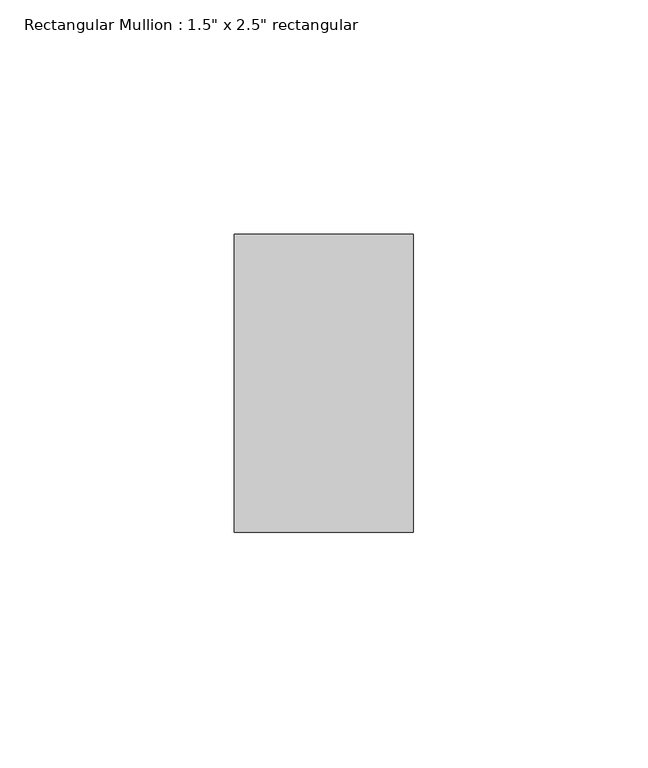
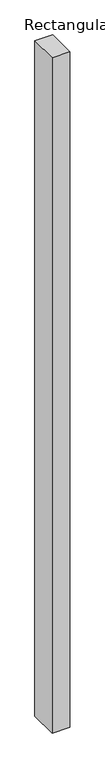
"""IFC4 building model written with IfcOpenShell, lengths in millimetres: member geometry."""

from ifc_helpers import new_model, si_unit, frame, origin, place, context, project, spatial, polyline, outline, extrude, source, transform, mapped, element, save


def member_155beb68(model_context):
    return source(origin(), model_context, "Body", "SweptSolid", [
        extrude(outline(polyline([(19.05, 31.75), (19.05, -31.75), (-19.05, -31.75), (-19.05, 31.75), (19.05, 31.75)])), frame((0.0, 0.0, -1524.0), z_axis=(0.0, 0.0, 1.0), x_axis=(1.0, 0.0, 0.0)), (0.0, 0.0, 1.0), 1524.0),
    ])


if __name__ == "__main__":
    model = new_model("IFC4")
    model_context = context("Model", 3, world=origin())
    ifc_project = project(units=[si_unit("LENGTHUNIT", "METRE", prefix="MILLI")], contexts=[model_context])
    site = spatial("IfcSite", under=ifc_project)
    building = spatial("IfcBuilding", under=site)
    placement = place(None, origin())
    member_shape = member_155beb68(model_context)
    element("IfcMember", 1, ObjectType="Rectangular Mullion : 1.5\" x 2.5\" rectangular", at=placement, inside=building, context=model_context, shape_type="MappedRepresentation", body=[
        mapped(member_shape, transform((0.0, 0.0, 0.0), x_axis=(1.0, 0.0, 0.0), y_axis=(0.0, 1.0, 0.0), z_axis=(0.0, 0.0, 1.0))),
    ])
    save(model, "model.ifc")

# Revit data of these elements
# Type "Rectangular Mullion : 1.5\" x 2.5\" rectangular"
#   built-in parameter 1007304 = 0.208333 (stored number, unit not read)
#   built-in parameter 1007301 = 0.0625 (stored number, unit not read)
#   built-in parameter 1007300 = 0.0625 (stored number, unit not read)
# Element 1 (IfcMember, "Rectangular Mullion : 1.5\" x 2.5\" rectangular")
#   Materials on its faces: "mullions"
# Materials
#   "mullions": class "Generic", colour RGB 120 120 120, transparency 0, Cost = 0
